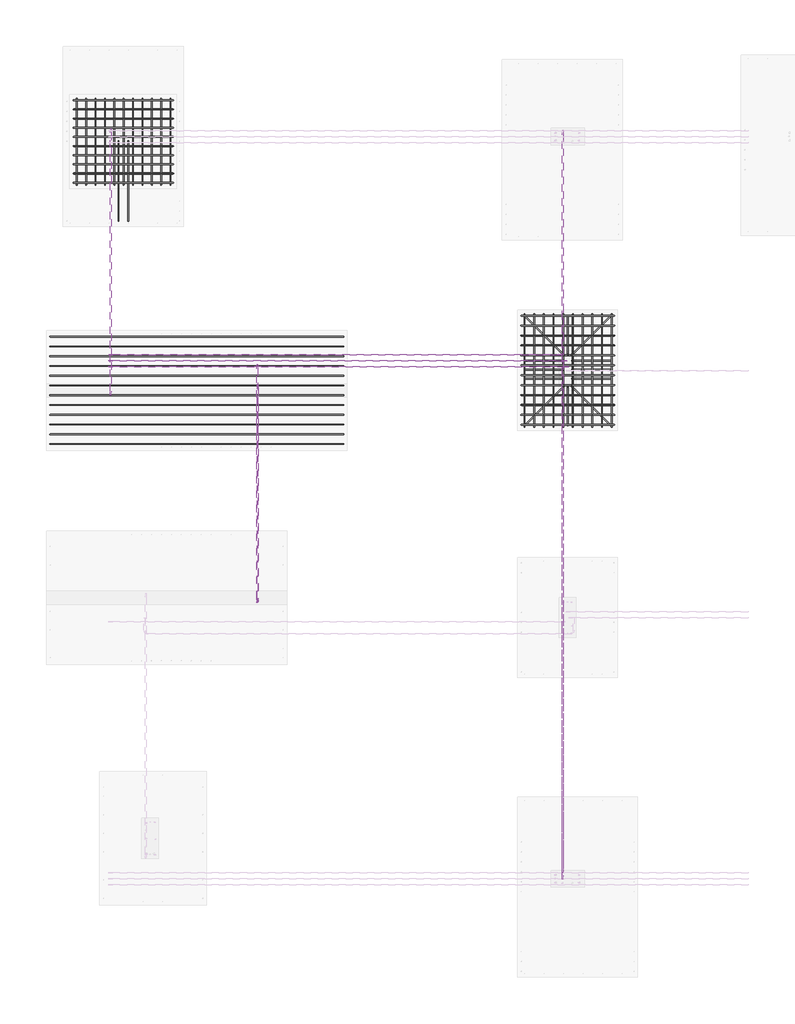
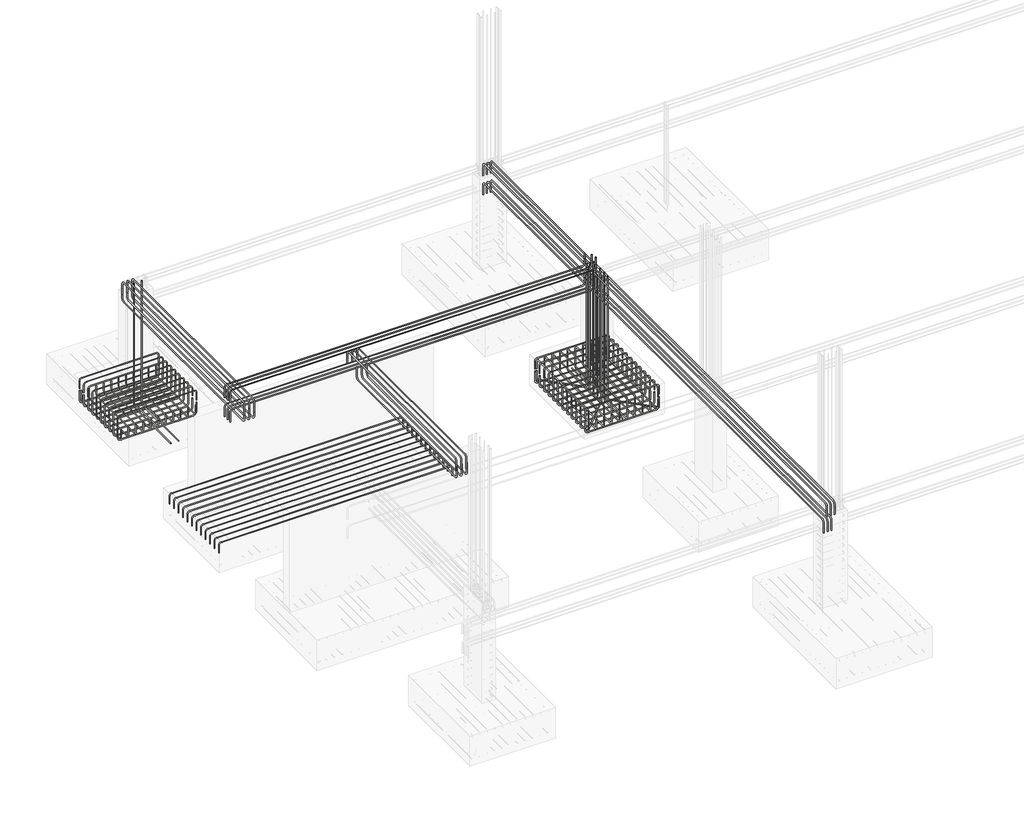
# One storey, part 11 of 18: 26 reinforcing bars.
"""IFC4 building model written with IfcOpenShell, lengths in millimetres."""

from ifc_helpers import new_model, si_unit, point, frame, origin, place, context, project, spatial, polyline, circle_curve, trimmed, segment, composite_curve, source, transform, mapped, element, save
from ifc_brep_helpers import swept_disk

model = new_model("IFC4")

# Units and contexts
model_context = context("Model", 3, world=origin())
ifc_project = project(units=[si_unit("LENGTHUNIT", "METRE", prefix="MILLI")], contexts=[model_context])

# Site, building, storey
site = spatial("IfcSite", under=ifc_project)
building = spatial("IfcBuilding", under=site)
storey = spatial("IfcBuildingStorey", under=building, Elevation=-2000.0)

# Reinforcing bars
placement = place(None, origin())
reinforcing_bar_shape = source(origin(), model_context, "Body", "SolidModel", [
    swept_disk(composite_curve([segment(polyline([(-14578.5790491, 6088.7024102, -2300.0), (-14578.5790491, 6088.7024102, -2486.6)]), True, "CONTINUOUS"), segment(trimmed(circle_curve(frame((-14634.0290491, 6088.7024102, -2486.6), z_axis=(0.0, 1.0, 0.0), x_axis=(55.44999999999891, 0.0, 0.0)), 55.45), [point((-14578.5790491, 6088.7024102, -2486.6))], [point((-14634.0290491, 6088.7024102, -2542.05))], True, "CARTESIAN"), True, "CONTINUOUS"), segment(polyline([(-14634.0290491, 6088.7024102, -2542.05), (-16007.2290491, 6088.7024102, -2542.05)]), True, "CONTINUOUS"), segment(trimmed(circle_curve(frame((-16007.2290491, 6088.7024102, -2486.6), z_axis=(0.0, 1.0, 0.0), x_axis=(0.0, 0.0, -55.45000000000027)), 55.45), [point((-16007.2290491, 6088.7024102, -2542.05))], [point((-16062.6790491, 6088.7024102, -2486.6))], True, "CARTESIAN"), True, "CONTINUOUS"), segment(polyline([(-16062.6790491, 6088.7024102, -2486.6), (-16062.6790491, 6088.7024102, -2300.0)]), True, "CONTINUOUS")], self_intersect=False), 7.95),
])
element("IfcReinforcingBar", 1, at=placement, inside=storey, context=model_context, shape_type="MappedRepresentation", body=[
    mapped(reinforcing_bar_shape, transform((0.0, 0.0, 0.0), x_axis=(1.0, 0.0, 0.0), y_axis=(0.0, 1.0, 0.0), z_axis=(0.0, 0.0, 1.0))),
    mapped(reinforcing_bar_shape, transform((0.0, -136.9639755, 0.0), x_axis=(1.0, 0.0, 0.0), y_axis=(0.0, 1.0, 0.0), z_axis=(0.0, 0.0, 1.0))),
    mapped(reinforcing_bar_shape, transform((0.0, -273.927951, 0.0), x_axis=(1.0, 0.0, 0.0), y_axis=(0.0, 1.0, 0.0), z_axis=(0.0, 0.0, 1.0))),
    mapped(reinforcing_bar_shape, transform((0.0, -410.8919265, 0.0), x_axis=(1.0, 0.0, 0.0), y_axis=(0.0, 1.0, 0.0), z_axis=(0.0, 0.0, 1.0))),
    mapped(reinforcing_bar_shape, transform((0.0, -547.8559021, 0.0), x_axis=(1.0, 0.0, 0.0), y_axis=(0.0, 1.0, 0.0), z_axis=(0.0, 0.0, 1.0))),
    mapped(reinforcing_bar_shape, transform((0.0, -684.8198776, 0.0), x_axis=(1.0, 0.0, 0.0), y_axis=(0.0, 1.0, 0.0), z_axis=(0.0, 0.0, 1.0))),
    mapped(reinforcing_bar_shape, transform((0.0, -821.7838531, 0.0), x_axis=(1.0, 0.0, 0.0), y_axis=(0.0, 1.0, 0.0), z_axis=(0.0, 0.0, 1.0))),
    mapped(reinforcing_bar_shape, transform((0.0, -958.7478286, 0.0), x_axis=(1.0, 0.0, 0.0), y_axis=(0.0, 1.0, 0.0), z_axis=(0.0, 0.0, 1.0))),
    mapped(reinforcing_bar_shape, transform((0.0, -1095.7118041, 0.0), x_axis=(1.0, 0.0, 0.0), y_axis=(0.0, 1.0, 0.0), z_axis=(0.0, 0.0, 1.0))),
    mapped(reinforcing_bar_shape, transform((0.0, -1232.6757796, 0.0), x_axis=(1.0, 0.0, 0.0), y_axis=(0.0, 1.0, 0.0), z_axis=(0.0, 0.0, 1.0))),
])
reinforcing_bar_2_shape = source(origin(), model_context, "Body", "SolidModel", [
    swept_disk(composite_curve([segment(polyline([(-16064.6290491, 6088.7024102, -2250.0), (-16064.6290491, 6088.7024102, -2102.0)]), True, "CONTINUOUS"), segment(trimmed(circle_curve(frame((-16018.6290491, 6088.7024102, -2102.0), z_axis=(0.0, 1.0, 0.0), x_axis=(-46.0, 0.0, 0.0)), 46.0), [point((-16064.6290491, 6088.7024102, -2102.0))], [point((-16018.6290491, 6088.7024102, -2056.0))], True, "CARTESIAN"), True, "CONTINUOUS"), segment(polyline([(-16018.6290491, 6088.7024102, -2056.0), (-14622.6290491, 6088.7024102, -2056.0)]), True, "CONTINUOUS"), segment(trimmed(circle_curve(frame((-14622.6290491, 6088.7024102, -2102.0), z_axis=(0.0, 1.0, 0.0), x_axis=(0.0, 0.0, 46.0)), 46.0), [point((-14622.6290491, 6088.7024102, -2056.0))], [point((-14576.6290491, 6088.7024102, -2102.0))], True, "CARTESIAN"), True, "CONTINUOUS"), segment(polyline([(-14576.6290491, 6088.7024102, -2102.0), (-14576.6290491, 6088.7024102, -2250.0)]), True, "CONTINUOUS")], self_intersect=False), 6.0),
])
element("IfcReinforcingBar", 2, at=placement, inside=storey, context=model_context, shape_type="MappedRepresentation", body=[
    mapped(reinforcing_bar_2_shape, transform((0.0, 0.0, 0.0), x_axis=(1.0, 0.0, 0.0), y_axis=(0.0, 1.0, 0.0), z_axis=(0.0, 0.0, 1.0))),
    mapped(reinforcing_bar_2_shape, transform((0.0, -136.9639755, 0.0), x_axis=(1.0, 0.0, 0.0), y_axis=(0.0, 1.0, 0.0), z_axis=(0.0, 0.0, 1.0))),
    mapped(reinforcing_bar_2_shape, transform((0.0, -273.927951, 0.0), x_axis=(1.0, 0.0, 0.0), y_axis=(0.0, 1.0, 0.0), z_axis=(0.0, 0.0, 1.0))),
    mapped(reinforcing_bar_2_shape, transform((0.0, -410.8919265, 0.0), x_axis=(1.0, 0.0, 0.0), y_axis=(0.0, 1.0, 0.0), z_axis=(0.0, 0.0, 1.0))),
    mapped(reinforcing_bar_2_shape, transform((0.0, -547.8559021, 0.0), x_axis=(1.0, 0.0, 0.0), y_axis=(0.0, 1.0, 0.0), z_axis=(0.0, 0.0, 1.0))),
    mapped(reinforcing_bar_2_shape, transform((0.0, -684.8198776, 0.0), x_axis=(1.0, 0.0, 0.0), y_axis=(0.0, 1.0, 0.0), z_axis=(0.0, 0.0, 1.0))),
    mapped(reinforcing_bar_2_shape, transform((0.0, -821.7838531, 0.0), x_axis=(1.0, 0.0, 0.0), y_axis=(0.0, 1.0, 0.0), z_axis=(0.0, 0.0, 1.0))),
    mapped(reinforcing_bar_2_shape, transform((0.0, -958.7478286, 0.0), x_axis=(1.0, 0.0, 0.0), y_axis=(0.0, 1.0, 0.0), z_axis=(0.0, 0.0, 1.0))),
    mapped(reinforcing_bar_2_shape, transform((0.0, -1095.7118041, 0.0), x_axis=(1.0, 0.0, 0.0), y_axis=(0.0, 1.0, 0.0), z_axis=(0.0, 0.0, 1.0))),
    mapped(reinforcing_bar_2_shape, transform((0.0, -1232.6757796, 0.0), x_axis=(1.0, 0.0, 0.0), y_axis=(0.0, 1.0, 0.0), z_axis=(0.0, 0.0, 1.0))),
])
reinforcing_bar_3_shape = source(origin(), model_context, "Body", "SolidModel", [
    swept_disk(composite_curve([segment(polyline([(-16018.4482662, 6111.5978854, -2322.6684255), (-16018.4482662, 6111.5978854, -2470.6684255)]), True, "CONTINUOUS"), segment(trimmed(circle_curve(frame((-16018.4482662, 6065.5978854, -2470.6684255), z_axis=(-1.0, 0.0, 0.0), x_axis=(0.0, 46.0, 0.0)), 46.0), [point((-16018.4482662, 6111.5978854, -2470.6684255))], [point((-16018.4482662, 6065.5978854, -2516.6684255))], True, "CARTESIAN"), True, "CONTINUOUS"), segment(polyline([(-16018.4482662, 6065.5978854, -2516.6684255), (-16018.4482662, 4869.5978854, -2516.6684255)]), True, "CONTINUOUS"), segment(trimmed(circle_curve(frame((-16018.4482662, 4869.5978854, -2470.6684255), z_axis=(-1.0, 0.0, 0.0), x_axis=(0.0, 0.0, -46.0)), 46.0), [point((-16018.4482662, 4869.5978854, -2516.6684255))], [point((-16018.4482662, 4823.5978854, -2470.6684255))], True, "CARTESIAN"), True, "CONTINUOUS"), segment(polyline([(-16018.4482662, 4823.5978854, -2470.6684255), (-16018.4482662, 4823.5978854, -2322.6684255)]), True, "CONTINUOUS")], self_intersect=False), 6.0),
])
element("IfcReinforcingBar", 3, at=placement, inside=storey, context=model_context, shape_type="MappedRepresentation", body=[
    mapped(reinforcing_bar_3_shape, transform((0.0, 0.0, 0.0), x_axis=(1.0, 0.0, 0.0), y_axis=(0.0, 1.0, 0.0), z_axis=(0.0, 0.0, 1.0))),
    mapped(reinforcing_bar_3_shape, transform((140.3819062, 0.0, 0.0), x_axis=(1.0, 0.0, 0.0), y_axis=(0.0, 1.0, 0.0), z_axis=(0.0, 0.0, 1.0))),
    mapped(reinforcing_bar_3_shape, transform((280.7638125, 0.0, 0.0), x_axis=(1.0, 0.0, 0.0), y_axis=(0.0, 1.0, 0.0), z_axis=(0.0, 0.0, 1.0))),
    mapped(reinforcing_bar_3_shape, transform((421.1457187, 0.0, 0.0), x_axis=(1.0, 0.0, 0.0), y_axis=(0.0, 1.0, 0.0), z_axis=(0.0, 0.0, 1.0))),
    mapped(reinforcing_bar_3_shape, transform((561.5276249, 0.0, 0.0), x_axis=(1.0, 0.0, 0.0), y_axis=(0.0, 1.0, 0.0), z_axis=(0.0, 0.0, 1.0))),
    mapped(reinforcing_bar_3_shape, transform((701.9095312, 0.0, 0.0), x_axis=(1.0, 0.0, 0.0), y_axis=(0.0, 1.0, 0.0), z_axis=(0.0, 0.0, 1.0))),
    mapped(reinforcing_bar_3_shape, transform((842.2914374, 0.0, 0.0), x_axis=(1.0, 0.0, 0.0), y_axis=(0.0, 1.0, 0.0), z_axis=(0.0, 0.0, 1.0))),
    mapped(reinforcing_bar_3_shape, transform((982.6733436, 0.0, 0.0), x_axis=(1.0, 0.0, 0.0), y_axis=(0.0, 1.0, 0.0), z_axis=(0.0, 0.0, 1.0))),
    mapped(reinforcing_bar_3_shape, transform((1123.0552499, 0.0, 0.0), x_axis=(1.0, 0.0, 0.0), y_axis=(0.0, 1.0, 0.0), z_axis=(0.0, 0.0, 1.0))),
    mapped(reinforcing_bar_3_shape, transform((1263.4371561, 0.0, 0.0), x_axis=(1.0, 0.0, 0.0), y_axis=(0.0, 1.0, 0.0), z_axis=(0.0, 0.0, 1.0))),
    mapped(reinforcing_bar_3_shape, transform((1403.8190623, 0.0, 0.0), x_axis=(1.0, 0.0, 0.0), y_axis=(0.0, 1.0, 0.0), z_axis=(0.0, 0.0, 1.0))),
])
reinforcing_bar_4_shape = source(origin(), model_context, "Body", "SolidModel", [
    swept_disk(composite_curve([segment(polyline([(-7979.5914888, 2865.1444872, -2300.0), (-7979.5914888, 2865.1444872, -2486.6)]), True, "CONTINUOUS"), segment(trimmed(circle_curve(frame((-8035.0414888, 2865.1444872, -2486.6), z_axis=(0.0, 1.0, 0.0), x_axis=(55.44999999999982, 0.0, 0.0)), 55.45), [point((-7979.5914888, 2865.1444872, -2486.6))], [point((-8035.0414888, 2865.1444872, -2542.05))], True, "CARTESIAN"), True, "CONTINUOUS"), segment(polyline([(-8035.0414888, 2865.1444872, -2542.05), (-9308.2414888, 2865.1444872, -2542.05)]), True, "CONTINUOUS"), segment(trimmed(circle_curve(frame((-9308.2414888, 2865.1444872, -2486.6), z_axis=(0.0, 1.0, 0.0), x_axis=(0.0, 0.0, -55.45000000000027)), 55.45), [point((-9308.2414888, 2865.1444872, -2542.05))], [point((-9363.6914888, 2865.1444872, -2486.6))], True, "CARTESIAN"), True, "CONTINUOUS"), segment(polyline([(-9363.6914888, 2865.1444872, -2486.6), (-9363.6914888, 2865.1444872, -2300.0)]), True, "CONTINUOUS")], self_intersect=False), 7.95),
])
element("IfcReinforcingBar", 4, at=placement, inside=storey, context=model_context, shape_type="MappedRepresentation", body=[
    mapped(reinforcing_bar_4_shape, transform((0.0, 0.0, 0.0), x_axis=(1.0, 0.0, 0.0), y_axis=(0.0, 1.0, 0.0), z_axis=(0.0, 0.0, 1.0))),
    mapped(reinforcing_bar_4_shape, transform((0.0, -148.4250709, 0.0), x_axis=(1.0, 0.0, 0.0), y_axis=(0.0, 1.0, 0.0), z_axis=(0.0, 0.0, 1.0))),
    mapped(reinforcing_bar_4_shape, transform((0.0, -296.8501418, 0.0), x_axis=(1.0, 0.0, 0.0), y_axis=(0.0, 1.0, 0.0), z_axis=(0.0, 0.0, 1.0))),
    mapped(reinforcing_bar_4_shape, transform((0.0, -445.2752126, 0.0), x_axis=(1.0, 0.0, 0.0), y_axis=(0.0, 1.0, 0.0), z_axis=(0.0, 0.0, 1.0))),
    mapped(reinforcing_bar_4_shape, transform((0.0, -593.7002835, 0.0), x_axis=(1.0, 0.0, 0.0), y_axis=(0.0, 1.0, 0.0), z_axis=(0.0, 0.0, 1.0))),
    mapped(reinforcing_bar_4_shape, transform((0.0, -742.1253544, 0.0), x_axis=(1.0, 0.0, 0.0), y_axis=(0.0, 1.0, 0.0), z_axis=(0.0, 0.0, 1.0))),
    mapped(reinforcing_bar_4_shape, transform((0.0, -890.5504253, 0.0), x_axis=(1.0, 0.0, 0.0), y_axis=(0.0, 1.0, 0.0), z_axis=(0.0, 0.0, 1.0))),
    mapped(reinforcing_bar_4_shape, transform((0.0, -1038.9754961, 0.0), x_axis=(1.0, 0.0, 0.0), y_axis=(0.0, 1.0, 0.0), z_axis=(0.0, 0.0, 1.0))),
    mapped(reinforcing_bar_4_shape, transform((0.0, -1187.400567, 0.0), x_axis=(1.0, 0.0, 0.0), y_axis=(0.0, 1.0, 0.0), z_axis=(0.0, 0.0, 1.0))),
    mapped(reinforcing_bar_4_shape, transform((0.0, -1335.8256379, 0.0), x_axis=(1.0, 0.0, 0.0), y_axis=(0.0, 1.0, 0.0), z_axis=(0.0, 0.0, 1.0))),
    mapped(reinforcing_bar_4_shape, transform((0.0, -1484.2507088, 0.0), x_axis=(1.0, 0.0, 0.0), y_axis=(0.0, 1.0, 0.0), z_axis=(0.0, 0.0, 1.0))),
    mapped(reinforcing_bar_4_shape, transform((0.0, -1632.6757796, 0.0), x_axis=(1.0, 0.0, 0.0), y_axis=(0.0, 1.0, 0.0), z_axis=(0.0, 0.0, 1.0))),
])
reinforcing_bar_5_shape = source(origin(), model_context, "Body", "SolidModel", [
    swept_disk(composite_curve([segment(polyline([(-9365.6414888, 2865.1444872, -2250.0), (-9365.6414888, 2865.1444872, -2102.0)]), True, "CONTINUOUS"), segment(trimmed(circle_curve(frame((-9319.6414888, 2865.1444872, -2102.0), z_axis=(0.0, 1.0, 0.0), x_axis=(-46.0, 0.0, 0.0)), 46.0), [point((-9365.6414888, 2865.1444872, -2102.0))], [point((-9319.6414888, 2865.1444872, -2056.0))], True, "CARTESIAN"), True, "CONTINUOUS"), segment(polyline([(-9319.6414888, 2865.1444872, -2056.0), (-8023.6414888, 2865.1444872, -2056.0)]), True, "CONTINUOUS"), segment(trimmed(circle_curve(frame((-8023.6414888, 2865.1444872, -2102.0), z_axis=(0.0, 1.0, 0.0), x_axis=(0.0, 0.0, 46.0)), 46.0), [point((-8023.6414888, 2865.1444872, -2056.0))], [point((-7977.6414888, 2865.1444872, -2102.0))], True, "CARTESIAN"), True, "CONTINUOUS"), segment(polyline([(-7977.6414888, 2865.1444872, -2102.0), (-7977.6414888, 2865.1444872, -2250.0)]), True, "CONTINUOUS")], self_intersect=False), 6.0),
])
element("IfcReinforcingBar", 5, at=placement, inside=storey, context=model_context, shape_type="MappedRepresentation", body=[
    mapped(reinforcing_bar_5_shape, transform((0.0, 0.0, 0.0), x_axis=(1.0, 0.0, 0.0), y_axis=(0.0, 1.0, 0.0), z_axis=(0.0, 0.0, 1.0))),
    mapped(reinforcing_bar_5_shape, transform((0.0, -148.4250709, 0.0), x_axis=(1.0, 0.0, 0.0), y_axis=(0.0, 1.0, 0.0), z_axis=(0.0, 0.0, 1.0))),
    mapped(reinforcing_bar_5_shape, transform((0.0, -296.8501418, 0.0), x_axis=(1.0, 0.0, 0.0), y_axis=(0.0, 1.0, 0.0), z_axis=(0.0, 0.0, 1.0))),
    mapped(reinforcing_bar_5_shape, transform((0.0, -445.2752126, 0.0), x_axis=(1.0, 0.0, 0.0), y_axis=(0.0, 1.0, 0.0), z_axis=(0.0, 0.0, 1.0))),
    mapped(reinforcing_bar_5_shape, transform((0.0, -593.7002835, 0.0), x_axis=(1.0, 0.0, 0.0), y_axis=(0.0, 1.0, 0.0), z_axis=(0.0, 0.0, 1.0))),
    mapped(reinforcing_bar_5_shape, transform((0.0, -742.1253544, 0.0), x_axis=(1.0, 0.0, 0.0), y_axis=(0.0, 1.0, 0.0), z_axis=(0.0, 0.0, 1.0))),
    mapped(reinforcing_bar_5_shape, transform((0.0, -890.5504253, 0.0), x_axis=(1.0, 0.0, 0.0), y_axis=(0.0, 1.0, 0.0), z_axis=(0.0, 0.0, 1.0))),
    mapped(reinforcing_bar_5_shape, transform((0.0, -1038.9754961, 0.0), x_axis=(1.0, 0.0, 0.0), y_axis=(0.0, 1.0, 0.0), z_axis=(0.0, 0.0, 1.0))),
    mapped(reinforcing_bar_5_shape, transform((0.0, -1187.400567, 0.0), x_axis=(1.0, 0.0, 0.0), y_axis=(0.0, 1.0, 0.0), z_axis=(0.0, 0.0, 1.0))),
    mapped(reinforcing_bar_5_shape, transform((0.0, -1335.8256379, 0.0), x_axis=(1.0, 0.0, 0.0), y_axis=(0.0, 1.0, 0.0), z_axis=(0.0, 0.0, 1.0))),
    mapped(reinforcing_bar_5_shape, transform((0.0, -1484.2507088, 0.0), x_axis=(1.0, 0.0, 0.0), y_axis=(0.0, 1.0, 0.0), z_axis=(0.0, 0.0, 1.0))),
    mapped(reinforcing_bar_5_shape, transform((0.0, -1632.6757796, 0.0), x_axis=(1.0, 0.0, 0.0), y_axis=(0.0, 1.0, 0.0), z_axis=(0.0, 0.0, 1.0))),
])
reinforcing_bar_6_shape = source(origin(), model_context, "Body", "SolidModel", [
    swept_disk(composite_curve([segment(polyline([(-9319.460706, 2888.0399624, -2322.6684255), (-9319.460706, 2888.0399624, -2470.6684255)]), True, "CONTINUOUS"), segment(trimmed(circle_curve(frame((-9319.460706, 2842.0399624, -2470.6684255), z_axis=(-1.0, 0.0, 0.0), x_axis=(0.0, 46.0, 0.0)), 46.0), [point((-9319.460706, 2888.0399624, -2470.6684255))], [point((-9319.460706, 2842.0399624, -2516.6684255))], True, "CARTESIAN"), True, "CONTINUOUS"), segment(polyline([(-9319.460706, 2842.0399624, -2516.6684255), (-9319.460706, 1246.0399624, -2516.6684255)]), True, "CONTINUOUS"), segment(trimmed(circle_curve(frame((-9319.460706, 1246.0399624, -2470.6684255), z_axis=(-1.0, 0.0, 0.0), x_axis=(0.0, 0.0, -46.0)), 46.0), [point((-9319.460706, 1246.0399624, -2516.6684255))], [point((-9319.460706, 1200.0399624, -2470.6684255))], True, "CARTESIAN"), True, "CONTINUOUS"), segment(polyline([(-9319.460706, 1200.0399624, -2470.6684255), (-9319.460706, 1200.0399624, -2322.6684255)]), True, "CONTINUOUS")], self_intersect=False), 6.0),
])
element("IfcReinforcingBar", 6, at=placement, inside=storey, context=model_context, shape_type="MappedRepresentation", body=[
    mapped(reinforcing_bar_6_shape, transform((0.0, 0.0, 0.0), x_axis=(1.0, 0.0, 0.0), y_axis=(0.0, 1.0, 0.0), z_axis=(0.0, 0.0, 1.0))),
    mapped(reinforcing_bar_6_shape, transform((144.8687847, 0.0, 0.0), x_axis=(1.0, 0.0, 0.0), y_axis=(0.0, 1.0, 0.0), z_axis=(0.0, 0.0, 1.0))),
    mapped(reinforcing_bar_6_shape, transform((289.7375694, 0.0, 0.0), x_axis=(1.0, 0.0, 0.0), y_axis=(0.0, 1.0, 0.0), z_axis=(0.0, 0.0, 1.0))),
    mapped(reinforcing_bar_6_shape, transform((434.6063541, 0.0, 0.0), x_axis=(1.0, 0.0, 0.0), y_axis=(0.0, 1.0, 0.0), z_axis=(0.0, 0.0, 1.0))),
    mapped(reinforcing_bar_6_shape, transform((579.4751388, 0.0, 0.0), x_axis=(1.0, 0.0, 0.0), y_axis=(0.0, 1.0, 0.0), z_axis=(0.0, 0.0, 1.0))),
    mapped(reinforcing_bar_6_shape, transform((724.3439235, 0.0, 0.0), x_axis=(1.0, 0.0, 0.0), y_axis=(0.0, 1.0, 0.0), z_axis=(0.0, 0.0, 1.0))),
    mapped(reinforcing_bar_6_shape, transform((869.2127082, 0.0, 0.0), x_axis=(1.0, 0.0, 0.0), y_axis=(0.0, 1.0, 0.0), z_axis=(0.0, 0.0, 1.0))),
    mapped(reinforcing_bar_6_shape, transform((1014.0814929, 0.0, 0.0), x_axis=(1.0, 0.0, 0.0), y_axis=(0.0, 1.0, 0.0), z_axis=(0.0, 0.0, 1.0))),
    mapped(reinforcing_bar_6_shape, transform((1158.9502776, 0.0, 0.0), x_axis=(1.0, 0.0, 0.0), y_axis=(0.0, 1.0, 0.0), z_axis=(0.0, 0.0, 1.0))),
    mapped(reinforcing_bar_6_shape, transform((1303.8190623, 0.0, 0.0), x_axis=(1.0, 0.0, 0.0), y_axis=(0.0, 1.0, 0.0), z_axis=(0.0, 0.0, 1.0))),
])
reinforcing_bar_7_shape = source(origin(), model_context, "Body", "SolidModel", [
    swept_disk(composite_curve([segment(polyline([(-8013.7184718, 2888.0399624, -2276.6677805), (-8013.7184718, 2888.0399624, -2128.6677805)]), True, "CONTINUOUS"), segment(trimmed(circle_curve(frame((-8013.7184718, 2842.0399624, -2128.6677805), z_axis=(1.0, 0.0, 0.0), x_axis=(0.0, 46.0, 0.0)), 46.0), [point((-8013.7184718, 2888.0399624, -2128.6677805))], [point((-8013.7184718, 2842.0399624, -2082.6677805))], True, "CARTESIAN"), True, "CONTINUOUS"), segment(polyline([(-8013.7184718, 2842.0399624, -2082.6677805), (-8013.7184718, 1246.0399624, -2082.6677805)]), True, "CONTINUOUS"), segment(trimmed(circle_curve(frame((-8013.7184718, 1246.0399624, -2128.6677805), z_axis=(1.0, 0.0, 0.0), x_axis=(0.0, 0.0, 46.0)), 46.0), [point((-8013.7184718, 1246.0399624, -2082.6677805))], [point((-8013.7184718, 1200.0399624, -2128.6677805))], True, "CARTESIAN"), True, "CONTINUOUS"), segment(polyline([(-8013.7184718, 1200.0399624, -2128.6677805), (-8013.7184718, 1200.0399624, -2276.6677805)]), True, "CONTINUOUS")], self_intersect=False), 6.0),
])
element("IfcReinforcingBar", 7, at=placement, inside=storey, context=model_context, shape_type="MappedRepresentation", body=[
    mapped(reinforcing_bar_7_shape, transform((0.0, 0.0, 0.0), x_axis=(1.0, 0.0, 0.0), y_axis=(0.0, 1.0, 0.0), z_axis=(0.0, 0.0, 1.0))),
    mapped(reinforcing_bar_7_shape, transform((-145.0824705, 0.0, 0.0), x_axis=(1.0, 0.0, 0.0), y_axis=(0.0, 1.0, 0.0), z_axis=(0.0, 0.0, 1.0))),
    mapped(reinforcing_bar_7_shape, transform((-290.1649409, 0.0, 0.0), x_axis=(1.0, 0.0, 0.0), y_axis=(0.0, 1.0, 0.0), z_axis=(0.0, 0.0, 1.0))),
    mapped(reinforcing_bar_7_shape, transform((-435.2474114, 0.0, 0.0), x_axis=(1.0, 0.0, 0.0), y_axis=(0.0, 1.0, 0.0), z_axis=(0.0, 0.0, 1.0))),
    mapped(reinforcing_bar_7_shape, transform((-580.3298819, 0.0, 0.0), x_axis=(1.0, 0.0, 0.0), y_axis=(0.0, 1.0, 0.0), z_axis=(0.0, 0.0, 1.0))),
    mapped(reinforcing_bar_7_shape, transform((-725.4123523, 0.0, 0.0), x_axis=(1.0, 0.0, 0.0), y_axis=(0.0, 1.0, 0.0), z_axis=(0.0, 0.0, 1.0))),
    mapped(reinforcing_bar_7_shape, transform((-870.4948228, 0.0, 0.0), x_axis=(1.0, 0.0, 0.0), y_axis=(0.0, 1.0, 0.0), z_axis=(0.0, 0.0, 1.0))),
    mapped(reinforcing_bar_7_shape, transform((-1015.5772932, 0.0, 0.0), x_axis=(1.0, 0.0, 0.0), y_axis=(0.0, 1.0, 0.0), z_axis=(0.0, 0.0, 1.0))),
    mapped(reinforcing_bar_7_shape, transform((-1160.6597637, 0.0, 0.0), x_axis=(1.0, 0.0, 0.0), y_axis=(0.0, 1.0, 0.0), z_axis=(0.0, 0.0, 1.0))),
    mapped(reinforcing_bar_7_shape, transform((-1305.7422342, 0.0, 0.0), x_axis=(1.0, 0.0, 0.0), y_axis=(0.0, 1.0, 0.0), z_axis=(0.0, 0.0, 1.0))),
])
reinforcing_bar_8_shape = source(origin(), model_context, "Body", "SolidModel", [
    swept_disk(composite_curve([segment(polyline([(-16414.5957341, 2550.5209024, -2276.6677805), (-16414.5957341, 2550.5209024, -2128.6677805)]), True, "CONTINUOUS"), segment(trimmed(circle_curve(frame((-16368.5957341, 2550.5209024, -2128.6677805), z_axis=(0.0, 1.0, 0.0), x_axis=(-46.0, 0.0, 0.0)), 46.0), [point((-16414.5957341, 2550.5209024, -2128.6677805))], [point((-16368.5957341, 2550.5209024, -2082.6677805))], True, "CARTESIAN"), True, "CONTINUOUS"), segment(polyline([(-16368.5957341, 2550.5209024, -2082.6677805), (-12074.5957341, 2550.5209024, -2082.6677805)]), True, "CONTINUOUS"), segment(trimmed(circle_curve(frame((-12074.5957341, 2550.5209024, -2128.6677805), z_axis=(0.0, 1.0, 0.0), x_axis=(0.0, 0.0, 46.0)), 46.0), [point((-12074.5957341, 2550.5209024, -2082.6677805))], [point((-12028.5957341, 2550.5209024, -2128.6677805))], True, "CARTESIAN"), True, "CONTINUOUS"), segment(polyline([(-12028.5957341, 2550.5209024, -2128.6677805), (-12028.5957341, 2550.5209024, -2276.6677805)]), True, "CONTINUOUS")], self_intersect=False), 6.0),
])
element("IfcReinforcingBar", 8, at=placement, inside=storey, context=model_context, shape_type="MappedRepresentation", body=[
    mapped(reinforcing_bar_8_shape, transform((0.0, 0.0, 0.0), x_axis=(1.0, 0.0, 0.0), y_axis=(0.0, 1.0, 0.0), z_axis=(0.0, 0.0, 1.0))),
    mapped(reinforcing_bar_8_shape, transform((0.0, -145.9765667, 0.0), x_axis=(1.0, 0.0, 0.0), y_axis=(0.0, 1.0, 0.0), z_axis=(0.0, 0.0, 1.0))),
    mapped(reinforcing_bar_8_shape, transform((0.0, -291.9531335, 0.0), x_axis=(1.0, 0.0, 0.0), y_axis=(0.0, 1.0, 0.0), z_axis=(0.0, 0.0, 1.0))),
    mapped(reinforcing_bar_8_shape, transform((0.0, -437.9297002, 0.0), x_axis=(1.0, 0.0, 0.0), y_axis=(0.0, 1.0, 0.0), z_axis=(0.0, 0.0, 1.0))),
    mapped(reinforcing_bar_8_shape, transform((0.0, -583.906267, 0.0), x_axis=(1.0, 0.0, 0.0), y_axis=(0.0, 1.0, 0.0), z_axis=(0.0, 0.0, 1.0))),
    mapped(reinforcing_bar_8_shape, transform((0.0, -729.8828337, 0.0), x_axis=(1.0, 0.0, 0.0), y_axis=(0.0, 1.0, 0.0), z_axis=(0.0, 0.0, 1.0))),
    mapped(reinforcing_bar_8_shape, transform((0.0, -875.8594005, 0.0), x_axis=(1.0, 0.0, 0.0), y_axis=(0.0, 1.0, 0.0), z_axis=(0.0, 0.0, 1.0))),
    mapped(reinforcing_bar_8_shape, transform((0.0, -1021.8359672, 0.0), x_axis=(1.0, 0.0, 0.0), y_axis=(0.0, 1.0, 0.0), z_axis=(0.0, 0.0, 1.0))),
    mapped(reinforcing_bar_8_shape, transform((0.0, -1167.8125339, 0.0), x_axis=(1.0, 0.0, 0.0), y_axis=(0.0, 1.0, 0.0), z_axis=(0.0, 0.0, 1.0))),
    mapped(reinforcing_bar_8_shape, transform((0.0, -1313.7891007, 0.0), x_axis=(1.0, 0.0, 0.0), y_axis=(0.0, 1.0, 0.0), z_axis=(0.0, 0.0, 1.0))),
    mapped(reinforcing_bar_8_shape, transform((0.0, -1459.7656674, 0.0), x_axis=(1.0, 0.0, 0.0), y_axis=(0.0, 1.0, 0.0), z_axis=(0.0, 0.0, 1.0))),
    mapped(reinforcing_bar_8_shape, transform((0.0, -1605.7422342, 0.0), x_axis=(1.0, 0.0, 0.0), y_axis=(0.0, 1.0, 0.0), z_axis=(0.0, 0.0, 1.0))),
])
reinforcing_bar_9_shape = source(origin(), model_context, "Body", "SolidModel", [
    swept_disk(composite_curve([segment(polyline([(-15393.6811441, 4281.0266306, -2480.0), (-15393.6811441, 5430.560053, -2480.0)]), True, "CONTINUOUS"), segment(trimmed(circle_curve(frame((-15393.6811441, 5430.560053, -2434.0), z_axis=(1.0, 0.0, 0.0), x_axis=(0.0, 0.0, -46.0)), 46.0), [point((-15393.6811441, 5430.560053, -2480.0))], [point((-15393.6811441, 5476.560053, -2434.0))], True, "CARTESIAN"), True, "CONTINUOUS"), segment(polyline([(-15393.6811441, 5476.560053, -2434.0), (-15393.6811441, 5476.560053, -30.0)]), True, "CONTINUOUS")], self_intersect=False), 6.0),
])
element("IfcReinforcingBar", 9, at=placement, inside=storey, context=model_context, shape_type="MappedRepresentation", body=[
    mapped(reinforcing_bar_9_shape, transform((0.0, 0.0, 0.0), x_axis=(1.0, 0.0, 0.0), y_axis=(0.0, 1.0, 0.0), z_axis=(0.0, 0.0, 1.0))),
    mapped(reinforcing_bar_9_shape, transform((144.9594019, 0.0, 0.0), x_axis=(1.0, 0.0, 0.0), y_axis=(0.0, 1.0, 0.0), z_axis=(0.0, 0.0, 1.0))),
])
element("IfcReinforcingBar", 10, at=placement, inside=storey, context=model_context, shape_type="SolidModel", body=[
    swept_disk(composite_curve([segment(polyline([(-8728.3359054, 2276.9160019, -30.0), (-8728.3359054, 2276.9160019, -2431.15)]), True, "CONTINUOUS"), segment(trimmed(circle_curve(frame((-8767.5449764, 2316.125073, -2431.15), z_axis=(0.70710678118655, 0.707106781186545, 0.0), x_axis=(39.20907100000113, -39.209071100000074, 0.0)), 55.45), [point((-8728.3359054, 2276.9160019, -2431.15))], [point((-8767.5449764, 2316.125073, -2486.6))], True, "CARTESIAN"), True, "CONTINUOUS"), segment(polyline([(-8767.5449764, 2316.125073, -2486.6), (-9313.39029, 2861.9703866, -2486.6)]), True, "CONTINUOUS")], self_intersect=False), 7.95),
])
element("IfcReinforcingBar", 11, at=placement, inside=storey, context=model_context, shape_type="SolidModel", body=[
    swept_disk(composite_curve([segment(polyline([(-8671.037887, 2281.5175403, -30.0), (-8671.037887, 2281.5175403, -2440.6)]), True, "CONTINUOUS"), segment(trimmed(circle_curve(frame((-8671.037887, 2327.5175403, -2440.6), z_axis=(1.0, 0.0, 0.0), x_axis=(0.0, -46.0, 0.0)), 46.0), [point((-8671.037887, 2281.5175403, -2440.6))], [point((-8671.037887, 2327.5175403, -2486.6))], True, "CARTESIAN"), True, "CONTINUOUS"), segment(polyline([(-8671.037887, 2327.5175403, -2486.6), (-8671.037887, 2865.1444872, -2486.6)]), True, "CONTINUOUS")], self_intersect=False), 6.0),
])
reinforcing_bar_10_shape = source(origin(), model_context, "Body", "SolidModel", [
    swept_disk(composite_curve([segment(polyline([(-8734.496625, 1923.4577701, -30.0), (-8734.496625, 1923.4577701, -2436.6982733)]), True, "CONTINUOUS"), segment(trimmed(circle_curve(frame((-8780.496625, 1923.4577701, -2436.6982733), z_axis=(0.0, 1.0, 0.0), x_axis=(46.0, 0.0, 0.0)), 46.0), [point((-8734.496625, 1923.4577701, -2436.6982733))], [point((-8780.496625, 1923.4577701, -2482.6982733))], True, "CARTESIAN"), True, "CONTINUOUS"), segment(polyline([(-8780.496625, 1923.4577701, -2482.6982733), (-9318.7783172, 1923.4577701, -2482.6982733)]), True, "CONTINUOUS")], self_intersect=False), 6.0),
])
element("IfcReinforcingBar", 12, at=placement, inside=storey, context=model_context, shape_type="MappedRepresentation", body=[
    mapped(reinforcing_bar_10_shape, transform((0.0, 0.0, 0.0), x_axis=(1.0, 0.0, 0.0), y_axis=(0.0, 1.0, 0.0), z_axis=(0.0, 0.0, 1.0))),
    mapped(reinforcing_bar_10_shape, transform((0.0, 134.2724138, 0.0), x_axis=(1.0, 0.0, 0.0), y_axis=(0.0, 1.0, 0.0), z_axis=(0.0, 0.0, 1.0))),
    mapped(reinforcing_bar_10_shape, transform((0.0, 268.5448277, 0.0), x_axis=(1.0, 0.0, 0.0), y_axis=(0.0, 1.0, 0.0), z_axis=(0.0, 0.0, 1.0))),
])
reinforcing_bar_11_shape = source(origin(), model_context, "Body", "SolidModel", [
    swept_disk(composite_curve([segment(polyline([(-8606.6833135, 1923.4577701, -30.0), (-8606.6833135, 1923.4577701, -2436.6982733)]), True, "CONTINUOUS"), segment(trimmed(circle_curve(frame((-8560.6833135, 1923.4577701, -2436.6982733), z_axis=(0.0, -1.0, 0.0), x_axis=(-46.0, 0.0, 0.0)), 46.0), [point((-8606.6833135, 1923.4577701, -2436.6982733))], [point((-8560.6833135, 1923.4577701, -2482.6982733))], True, "CARTESIAN"), True, "CONTINUOUS"), segment(polyline([(-8560.6833135, 1923.4577701, -2482.6982733), (-8022.4016213, 1923.4577701, -2482.6982733)]), True, "CONTINUOUS")], self_intersect=False), 6.0),
])
element("IfcReinforcingBar", 13, at=placement, inside=storey, context=model_context, shape_type="MappedRepresentation", body=[
    mapped(reinforcing_bar_11_shape, transform((0.0, 0.0, 0.0), x_axis=(1.0, 0.0, 0.0), y_axis=(0.0, 1.0, 0.0), z_axis=(0.0, 0.0, 1.0))),
    mapped(reinforcing_bar_11_shape, transform((0.0, 134.2724138, 0.0), x_axis=(1.0, 0.0, 0.0), y_axis=(0.0, 1.0, 0.0), z_axis=(0.0, 0.0, 1.0))),
    mapped(reinforcing_bar_11_shape, transform((0.0, 268.5448277, 0.0), x_axis=(1.0, 0.0, 0.0), y_axis=(0.0, 1.0, 0.0), z_axis=(0.0, 0.0, 1.0))),
])
element("IfcReinforcingBar", 14, at=placement, inside=storey, context=model_context, shape_type="SolidModel", body=[
    swept_disk(composite_curve([segment(polyline([(-8671.037887, 1803.6782305, -30.0), (-8671.037887, 1803.6782305, -2440.6)]), True, "CONTINUOUS"), segment(trimmed(circle_curve(frame((-8671.037887, 1757.6782305, -2440.6), z_axis=(-1.0, 0.0, 0.0), x_axis=(0.0, 46.0, 0.0)), 46.0), [point((-8671.037887, 1803.6782305, -2440.6))], [point((-8671.037887, 1757.6782305, -2486.6))], True, "CARTESIAN"), True, "CONTINUOUS"), segment(polyline([(-8671.037887, 1757.6782305, -2486.6), (-8671.037887, 1220.0512836, -2486.6)]), True, "CONTINUOUS")], self_intersect=False), 6.0),
])
element("IfcReinforcingBar", 15, at=placement, inside=storey, context=model_context, shape_type="SolidModel", body=[
    swept_disk(composite_curve([segment(polyline([(-8612.8440331, 2276.9160019, -30.0), (-8612.8440331, 2276.9160019, -2431.15)]), True, "CONTINUOUS"), segment(trimmed(circle_curve(frame((-8573.634962, 2316.125073, -2431.15), z_axis=(0.70710678118655, -0.707106781186545, 0.0), x_axis=(-39.209071100000074, -39.209071100000074, 0.0)), 55.45), [point((-8612.8440331, 2276.9160019, -2431.15))], [point((-8573.634962, 2316.125073, -2486.6))], True, "CARTESIAN"), True, "CONTINUOUS"), segment(polyline([(-8573.634962, 2316.125073, -2486.6), (-8027.7896484, 2861.9703866, -2486.6)]), True, "CONTINUOUS")], self_intersect=False), 7.95),
])
element("IfcReinforcingBar", 16, at=placement, inside=storey, context=model_context, shape_type="SolidModel", body=[
    swept_disk(composite_curve([segment(polyline([(-8728.3359054, 1808.2797689, -30.0), (-8728.3359054, 1808.2797689, -2431.15)]), True, "CONTINUOUS"), segment(trimmed(circle_curve(frame((-8767.5449764, 1769.0706979, -2431.15), z_axis=(-0.7071067811865454, 0.7071067811865497, 0.0), x_axis=(39.20907100000113, 39.209070999999994, 0.0)), 55.45), [point((-8728.3359054, 1808.2797689, -2431.15))], [point((-8767.5449764, 1769.0706979, -2486.6))], True, "CARTESIAN"), True, "CONTINUOUS"), segment(polyline([(-8767.5449764, 1769.0706979, -2486.6), (-9313.39029, 1223.2253842, -2486.6)]), True, "CONTINUOUS")], self_intersect=False), 7.95),
])
element("IfcReinforcingBar", 17, at=placement, inside=storey, context=model_context, shape_type="SolidModel", body=[
    swept_disk(composite_curve([segment(polyline([(-8612.8440331, 1808.2797689, -30.0), (-8612.8440331, 1808.2797689, -2431.15)]), True, "CONTINUOUS"), segment(trimmed(circle_curve(frame((-8573.634962, 1769.0706979, -2431.15), z_axis=(-0.7071067811865545, -0.7071067811865406, 0.0), x_axis=(-39.209071100000074, 39.209070999999994, 0.0)), 55.45), [point((-8612.8440331, 1808.2797689, -2431.15))], [point((-8573.634962, 1769.0706979, -2486.6))], True, "CARTESIAN"), True, "CONTINUOUS"), segment(polyline([(-8573.634962, 1769.0706979, -2486.6), (-8027.7896484, 1223.2253842, -2486.6)]), True, "CONTINUOUS")], self_intersect=False), 7.95),
])
reinforcing_bar_12_shape = source(origin(), model_context, "Body", "SolidModel", [
    swept_disk(composite_curve([segment(polyline([(-15510.0194098, 1680.5478854, -300.05), (-15510.0194098, 1680.5478854, -113.45)]), True, "CONTINUOUS"), segment(trimmed(circle_curve(frame((-15510.0194098, 1735.9978854, -113.45), z_axis=(-1.0, 0.0, 0.0), x_axis=(0.0, -55.450000000000045, 0.0)), 55.45), [point((-15510.0194098, 1680.5478854, -113.45))], [point((-15510.0194098, 1735.9978854, -58.0))], True, "CARTESIAN"), True, "CONTINUOUS"), segment(polyline([(-15510.0194098, 1735.9978854, -58.0), (-15510.0194098, 5599.1978854, -58.0)]), True, "CONTINUOUS"), segment(trimmed(circle_curve(frame((-15510.0194098, 5599.1978854, -113.45), z_axis=(-1.0, 0.0, 0.0), x_axis=(0.0, 0.0, 55.45)), 55.45), [point((-15510.0194098, 5599.1978854, -58.0))], [point((-15510.0194098, 5654.6478854, -113.45))], True, "CARTESIAN"), True, "CONTINUOUS"), segment(polyline([(-15510.0194098, 5654.6478854, -113.45), (-15510.0194098, 5654.6478854, -300.05)]), True, "CONTINUOUS")], self_intersect=False), 7.95),
])
element("IfcReinforcingBar", 18, at=placement, inside=storey, context=model_context, shape_type="MappedRepresentation", body=[
    mapped(reinforcing_bar_12_shape, transform((0.0, 0.0, 0.0), x_axis=(1.0, 0.0, 0.0), y_axis=(0.0, 1.0, 0.0), z_axis=(0.0, 0.0, 1.0))),
    mapped(reinforcing_bar_12_shape, transform((90.514926, 0.0, 0.0), x_axis=(1.0, 0.0, 0.0), y_axis=(0.0, 1.0, 0.0), z_axis=(0.0, 0.0, 1.0))),
    mapped(reinforcing_bar_12_shape, transform((181.029852, 0.0, 0.0), x_axis=(1.0, 0.0, 0.0), y_axis=(0.0, 1.0, 0.0), z_axis=(0.0, 0.0, 1.0))),
])
reinforcing_bar_13_shape = source(origin(), model_context, "Body", "SolidModel", [
    swept_disk(composite_curve([segment(polyline([(-15510.0194098, 1680.5478854, -195.95), (-15510.0194098, 1680.5478854, -382.55)]), True, "CONTINUOUS"), segment(trimmed(circle_curve(frame((-15510.0194098, 1735.9978854, -382.55), z_axis=(1.0, 0.0, 0.0), x_axis=(0.0, -55.450000000000045, 0.0)), 55.45), [point((-15510.0194098, 1680.5478854, -382.55))], [point((-15510.0194098, 1735.9978854, -438.0))], True, "CARTESIAN"), True, "CONTINUOUS"), segment(polyline([(-15510.0194098, 1735.9978854, -438.0), (-15510.0194098, 5599.1978854, -438.0)]), True, "CONTINUOUS"), segment(trimmed(circle_curve(frame((-15510.0194098, 5599.1978854, -382.55), z_axis=(1.0, 0.0, 0.0), x_axis=(0.0, 0.0, -55.44999999999999)), 55.45), [point((-15510.0194098, 5599.1978854, -438.0))], [point((-15510.0194098, 5654.6478854, -382.55))], True, "CARTESIAN"), True, "CONTINUOUS"), segment(polyline([(-15510.0194098, 5654.6478854, -382.55), (-15510.0194098, 5654.6478854, -195.95)]), True, "CONTINUOUS")], self_intersect=False), 7.95),
])
element("IfcReinforcingBar", 19, at=placement, inside=storey, context=model_context, shape_type="MappedRepresentation", body=[
    mapped(reinforcing_bar_13_shape, transform((0.0, 0.0, 0.0), x_axis=(1.0, 0.0, 0.0), y_axis=(0.0, 1.0, 0.0), z_axis=(0.0, 0.0, 1.0))),
    mapped(reinforcing_bar_13_shape, transform((90.514926, 0.0, 0.0), x_axis=(1.0, 0.0, 0.0), y_axis=(0.0, 1.0, 0.0), z_axis=(0.0, 0.0, 1.0))),
    mapped(reinforcing_bar_13_shape, transform((181.029852, 0.0, 0.0), x_axis=(1.0, 0.0, 0.0), y_axis=(0.0, 1.0, 0.0), z_axis=(0.0, 0.0, 1.0))),
])
reinforcing_bar_14_shape = source(origin(), model_context, "Body", "SolidModel", [
    swept_disk(composite_curve([segment(polyline([(-8744.6461398, -5560.4633571, -297.9938294), (-8744.6461398, -5560.4633571, -111.3938294)]), True, "CONTINUOUS"), segment(trimmed(circle_curve(frame((-8744.6461398, -5505.0133571, -111.3938294), z_axis=(-1.0, 0.0, 0.0), x_axis=(0.0, -55.45000000000073, 0.0)), 55.45), [point((-8744.6461398, -5560.4633571, -111.3938294))], [point((-8744.6461398, -5505.0133571, -55.9438294))], True, "CARTESIAN"), True, "CONTINUOUS"), segment(polyline([(-8744.6461398, -5505.0133571, -55.9438294), (-8744.6461398, 5574.1978854, -55.9438294)]), True, "CONTINUOUS"), segment(trimmed(circle_curve(frame((-8744.6461398, 5574.1978854, -111.3938294), z_axis=(-1.0, 0.0, 0.0), x_axis=(0.0, 0.0, 55.45)), 55.45), [point((-8744.6461398, 5574.1978854, -55.9438294))], [point((-8744.6461398, 5629.6478854, -111.3938294))], True, "CARTESIAN"), True, "CONTINUOUS"), segment(polyline([(-8744.6461398, 5629.6478854, -111.3938294), (-8744.6461398, 5629.6478854, -297.9938294)]), True, "CONTINUOUS")], self_intersect=False), 7.95),
])
element("IfcReinforcingBar", 20, at=placement, inside=storey, context=model_context, shape_type="MappedRepresentation", body=[
    mapped(reinforcing_bar_14_shape, transform((0.0, 0.0, 0.0), x_axis=(1.0, 0.0, 0.0), y_axis=(0.0, 1.0, 0.0), z_axis=(0.0, 0.0, 1.0))),
    mapped(reinforcing_bar_14_shape, transform((72.4937066, 0.0, 0.0), x_axis=(1.0, 0.0, 0.0), y_axis=(0.0, 1.0, 0.0), z_axis=(0.0, 0.0, 1.0))),
    mapped(reinforcing_bar_14_shape, transform((144.9874132, 0.0, 0.0), x_axis=(1.0, 0.0, 0.0), y_axis=(0.0, 1.0, 0.0), z_axis=(0.0, 0.0, 1.0))),
])
reinforcing_bar_15_shape = source(origin(), model_context, "Body", "SolidModel", [
    swept_disk(composite_curve([segment(polyline([(-8744.6461398, -5458.7297656, -677.9938294), (-8744.6461398, -5458.7297656, -491.3938294)]), True, "CONTINUOUS"), segment(trimmed(circle_curve(frame((-8744.6461398, -5403.2797656, -491.3938294), z_axis=(-1.0, 0.0, 0.0), x_axis=(0.0, -55.44999999999982, 0.0)), 55.45), [point((-8744.6461398, -5458.7297656, -491.3938294))], [point((-8744.6461398, -5403.2797656, -435.9438294))], True, "CARTESIAN"), True, "CONTINUOUS"), segment(polyline([(-8744.6461398, -5403.2797656, -435.9438294), (-8744.6461398, 5574.1978854, -435.9438294)]), True, "CONTINUOUS"), segment(trimmed(circle_curve(frame((-8744.6461398, 5574.1978854, -491.3938294), z_axis=(-1.0, 0.0, 0.0), x_axis=(0.0, 0.0, 55.44999999999999)), 55.45), [point((-8744.6461398, 5574.1978854, -435.9438294))], [point((-8744.6461398, 5629.6478854, -491.3938294))], True, "CARTESIAN"), True, "CONTINUOUS"), segment(polyline([(-8744.6461398, 5629.6478854, -491.3938294), (-8744.6461398, 5629.6478854, -677.9938294)]), True, "CONTINUOUS")], self_intersect=False), 7.95),
])
element("IfcReinforcingBar", 21, at=placement, inside=storey, context=model_context, shape_type="MappedRepresentation", body=[
    mapped(reinforcing_bar_15_shape, transform((0.0, 0.0, 0.0), x_axis=(1.0, 0.0, 0.0), y_axis=(0.0, 1.0, 0.0), z_axis=(0.0, 0.0, 1.0))),
    mapped(reinforcing_bar_15_shape, transform((72.4937066, 0.0, 0.0), x_axis=(1.0, 0.0, 0.0), y_axis=(0.0, 1.0, 0.0), z_axis=(0.0, 0.0, 1.0))),
    mapped(reinforcing_bar_15_shape, transform((144.9874132, 0.0, 0.0), x_axis=(1.0, 0.0, 0.0), y_axis=(0.0, 1.0, 0.0), z_axis=(0.0, 0.0, 1.0))),
])
reinforcing_bar_16_shape = source(origin(), model_context, "Body", "SolidModel", [
    swept_disk(composite_curve([segment(polyline([(-13130.1207309, -1419.4521146, -300.05), (-13130.1207309, -1419.4521146, -113.45)]), True, "CONTINUOUS"), segment(trimmed(circle_curve(frame((-13130.1207309, -1364.0021146, -113.45), z_axis=(-1.0, 0.0, 0.0), x_axis=(0.0, -55.450000000000045, 0.0)), 55.45), [point((-13130.1207309, -1419.4521146, -113.45))], [point((-13130.1207309, -1364.0021146, -58.0))], True, "CARTESIAN"), True, "CONTINUOUS"), segment(polyline([(-13130.1207309, -1364.0021146, -58.0), (-13130.1207309, 2074.1978854, -58.0)]), True, "CONTINUOUS"), segment(trimmed(circle_curve(frame((-13130.1207309, 2074.1978854, -113.45), z_axis=(-1.0, 0.0, 0.0), x_axis=(0.0, 0.0, 55.45)), 55.45), [point((-13130.1207309, 2074.1978854, -58.0))], [point((-13130.1207309, 2129.6478854, -113.45))], True, "CARTESIAN"), True, "CONTINUOUS"), segment(polyline([(-13130.1207309, 2129.6478854, -113.45), (-13130.1207309, 2129.6478854, -300.05)]), True, "CONTINUOUS")], self_intersect=False), 7.95),
])
element("IfcReinforcingBar", 22, at=placement, inside=storey, context=model_context, shape_type="MappedRepresentation", body=[
    mapped(reinforcing_bar_16_shape, transform((0.0, 0.0, 0.0), x_axis=(1.0, 0.0, 0.0), y_axis=(0.0, 1.0, 0.0), z_axis=(0.0, 0.0, 1.0))),
    mapped(reinforcing_bar_16_shape, transform((-95.0506605, 0.0, 0.0), x_axis=(1.0, 0.0, 0.0), y_axis=(0.0, 1.0, 0.0), z_axis=(0.0, 0.0, 1.0))),
    mapped(reinforcing_bar_16_shape, transform((-190.1013211, 0.0, 0.0), x_axis=(1.0, 0.0, 0.0), y_axis=(0.0, 1.0, 0.0), z_axis=(0.0, 0.0, 1.0))),
])
reinforcing_bar_17_shape = source(origin(), model_context, "Body", "SolidModel", [
    swept_disk(composite_curve([segment(polyline([(-13310.222052, -1419.4521146, -207.0061706), (-13310.222052, -1419.4521146, -393.6061706)]), True, "CONTINUOUS"), segment(trimmed(circle_curve(frame((-13310.222052, -1364.0021146, -393.6061706), z_axis=(1.0, 0.0, 0.0), x_axis=(0.0, -55.450000000000045, 0.0)), 55.45), [point((-13310.222052, -1419.4521146, -393.6061706))], [point((-13310.222052, -1364.0021146, -449.0561706))], True, "CARTESIAN"), True, "CONTINUOUS"), segment(polyline([(-13310.222052, -1364.0021146, -449.0561706), (-13310.222052, 1774.1978854, -449.0561706)]), True, "CONTINUOUS"), segment(trimmed(circle_curve(frame((-13310.222052, 1774.1978854, -393.6061706), z_axis=(1.0, 0.0, 0.0), x_axis=(0.0, 0.0, -55.44999999999999)), 55.45), [point((-13310.222052, 1774.1978854, -449.0561706))], [point((-13310.222052, 1829.6478854, -393.6061706))], True, "CARTESIAN"), True, "CONTINUOUS"), segment(polyline([(-13310.222052, 1829.6478854, -393.6061706), (-13310.222052, 1829.6478854, -207.0061706)]), True, "CONTINUOUS")], self_intersect=False), 7.95),
])
element("IfcReinforcingBar", 23, at=placement, inside=storey, context=model_context, shape_type="MappedRepresentation", body=[
    mapped(reinforcing_bar_17_shape, transform((0.0, 0.0, 0.0), x_axis=(1.0, 0.0, 0.0), y_axis=(0.0, 1.0, 0.0), z_axis=(0.0, 0.0, 1.0))),
    mapped(reinforcing_bar_17_shape, transform((94.3245868, 0.0, 0.0), x_axis=(1.0, 0.0, 0.0), y_axis=(0.0, 1.0, 0.0), z_axis=(0.0, 0.0, 1.0))),
    mapped(reinforcing_bar_17_shape, transform((188.6491736, 0.0, 0.0), x_axis=(1.0, 0.0, 0.0), y_axis=(0.0, 1.0, 0.0), z_axis=(0.0, 0.0, 1.0))),
])
reinforcing_bar_18_shape = source(origin(), model_context, "Body", "SolidModel", [
    swept_disk(composite_curve([segment(polyline([(-15532.6790491, 2101.8478854, -300.2534207), (-15532.6790491, 2101.8478854, -113.6534207)]), True, "CONTINUOUS"), segment(trimmed(circle_curve(frame((-15477.2290491, 2101.8478854, -113.6534207), z_axis=(0.0, 1.0, 0.0), x_axis=(-55.44999999999891, 0.0, 0.0)), 55.45), [point((-15532.6790491, 2101.8478854, -113.6534207))], [point((-15477.2290491, 2101.8478854, -58.2034207))], True, "CARTESIAN"), True, "CONTINUOUS"), segment(polyline([(-15477.2290491, 2101.8478854, -58.2034207), (-8722.7101161, 2101.8478854, -58.2034207)]), True, "CONTINUOUS"), segment(trimmed(circle_curve(frame((-8722.7101161, 2101.8478854, -2.7534207), z_axis=(0.0, -1.0, 0.0), x_axis=(0.0, 0.0, -55.45)), 55.45), [point((-8722.7101161, 2101.8478854, -58.2034207))], [point((-8667.2601161, 2101.8478854, -2.7534207))], True, "CARTESIAN"), True, "CONTINUOUS"), segment(polyline([(-8667.2601161, 2101.8478854, -2.7534207), (-8667.2601161, 2101.8478854, 183.8465793)]), True, "CONTINUOUS")], self_intersect=False), 7.95),
])
element("IfcReinforcingBar", 24, at=placement, inside=storey, context=model_context, shape_type="MappedRepresentation", body=[
    mapped(reinforcing_bar_18_shape, transform((0.0, 0.0, 0.0), x_axis=(1.0, 0.0, 0.0), y_axis=(0.0, 1.0, 0.0), z_axis=(0.0, 0.0, 1.0))),
    mapped(reinforcing_bar_18_shape, transform((0.0, 0.0, -384.9941108), x_axis=(1.0, 0.0, 0.0), y_axis=(0.0, 1.0, 0.0), z_axis=(0.0, 0.0, 1.0))),
])
reinforcing_bar_19_shape = source(origin(), model_context, "Body", "SolidModel", [
    swept_disk(composite_curve([segment(polyline([(-15532.6790491, 2190.0978854, -300.2534207), (-15532.6790491, 2190.0978854, -113.6534207)]), True, "CONTINUOUS"), segment(trimmed(circle_curve(frame((-15477.2290491, 2190.0978854, -113.6534207), z_axis=(0.0, 1.0, 0.0), x_axis=(-55.44999999999891, 0.0, 0.0)), 55.45), [point((-15532.6790491, 2190.0978854, -113.6534207))], [point((-15477.2290491, 2190.0978854, -58.2034207))], True, "CARTESIAN"), True, "CONTINUOUS"), segment(polyline([(-15477.2290491, 2190.0978854, -58.2034207), (-8746.9627235, 2190.0978854, -58.2034207)]), True, "CONTINUOUS"), segment(trimmed(circle_curve(frame((-8746.9627235, 2190.0978854, -2.7534207), z_axis=(0.0, -1.0, 0.0), x_axis=(0.0, 0.0, -55.45)), 55.45), [point((-8746.9627235, 2190.0978854, -58.2034207))], [point((-8691.5127235, 2190.0978854, -2.7534207))], True, "CARTESIAN"), True, "CONTINUOUS"), segment(polyline([(-8691.5127235, 2190.0978854, -2.7534207), (-8691.5127235, 2190.0978854, 183.8465793)]), True, "CONTINUOUS")], self_intersect=False), 7.95),
])
element("IfcReinforcingBar", 25, at=placement, inside=storey, context=model_context, shape_type="MappedRepresentation", body=[
    mapped(reinforcing_bar_19_shape, transform((0.0, 0.0, 0.0), x_axis=(1.0, 0.0, 0.0), y_axis=(0.0, 1.0, 0.0), z_axis=(0.0, 0.0, 1.0))),
    mapped(reinforcing_bar_19_shape, transform((0.0, 0.0, -384.9941108), x_axis=(1.0, 0.0, 0.0), y_axis=(0.0, 1.0, 0.0), z_axis=(0.0, 0.0, 1.0))),
])
reinforcing_bar_20_shape = source(origin(), model_context, "Body", "SolidModel", [
    swept_disk(composite_curve([segment(polyline([(-15532.6790491, 2282.5978854, -303.2034207), (-15532.6790491, 2282.5978854, -116.6034207)]), True, "CONTINUOUS"), segment(trimmed(circle_curve(frame((-15477.2290491, 2282.5978854, -116.6034207), z_axis=(0.0, 1.0, 0.0), x_axis=(-55.44999999999891, 0.0, 0.0)), 55.45), [point((-15532.6790491, 2282.5978854, -116.6034207))], [point((-15477.2290491, 2282.5978854, -61.1534207))], True, "CARTESIAN"), True, "CONTINUOUS"), segment(polyline([(-15477.2290491, 2282.5978854, -61.1534207), (-8826.4945848, 2282.5978854, -61.1534207)]), True, "CONTINUOUS"), segment(trimmed(circle_curve(frame((-8826.4945848, 2282.5978854, -5.7034207), z_axis=(0.0, -1.0, 0.0), x_axis=(0.0, 0.0, -55.449999999999996)), 55.45), [point((-8826.4945848, 2282.5978854, -61.1534207))], [point((-8771.0445848, 2282.5978854, -5.7034207))], True, "CARTESIAN"), True, "CONTINUOUS"), segment(polyline([(-8771.0445848, 2282.5978854, -5.7034207), (-8771.0445848, 2282.5978854, 180.8965793)]), True, "CONTINUOUS")], self_intersect=False), 7.95),
])
element("IfcReinforcingBar", 26, at=placement, inside=storey, context=model_context, shape_type="MappedRepresentation", body=[
    mapped(reinforcing_bar_20_shape, transform((0.0, 0.0, 0.0), x_axis=(1.0, 0.0, 0.0), y_axis=(0.0, 1.0, 0.0), z_axis=(0.0, 0.0, 1.0))),
    mapped(reinforcing_bar_20_shape, transform((0.0, 0.0, -384.9941108), x_axis=(1.0, 0.0, 0.0), y_axis=(0.0, 1.0, 0.0), z_axis=(0.0, 0.0, 1.0))),
])

save(model, "model.ifc")

# Revit data of these elements
# Elements 1, 2, 3, 4, 5, 6, 7, 8, 9, 10, 11, 12, 13, 14, 15, 16, 17, 18, 19, 20, 21, 22, 23, 24, 25, 26 (IfcReinforcingBar)
#   Phase Created = New Construction
